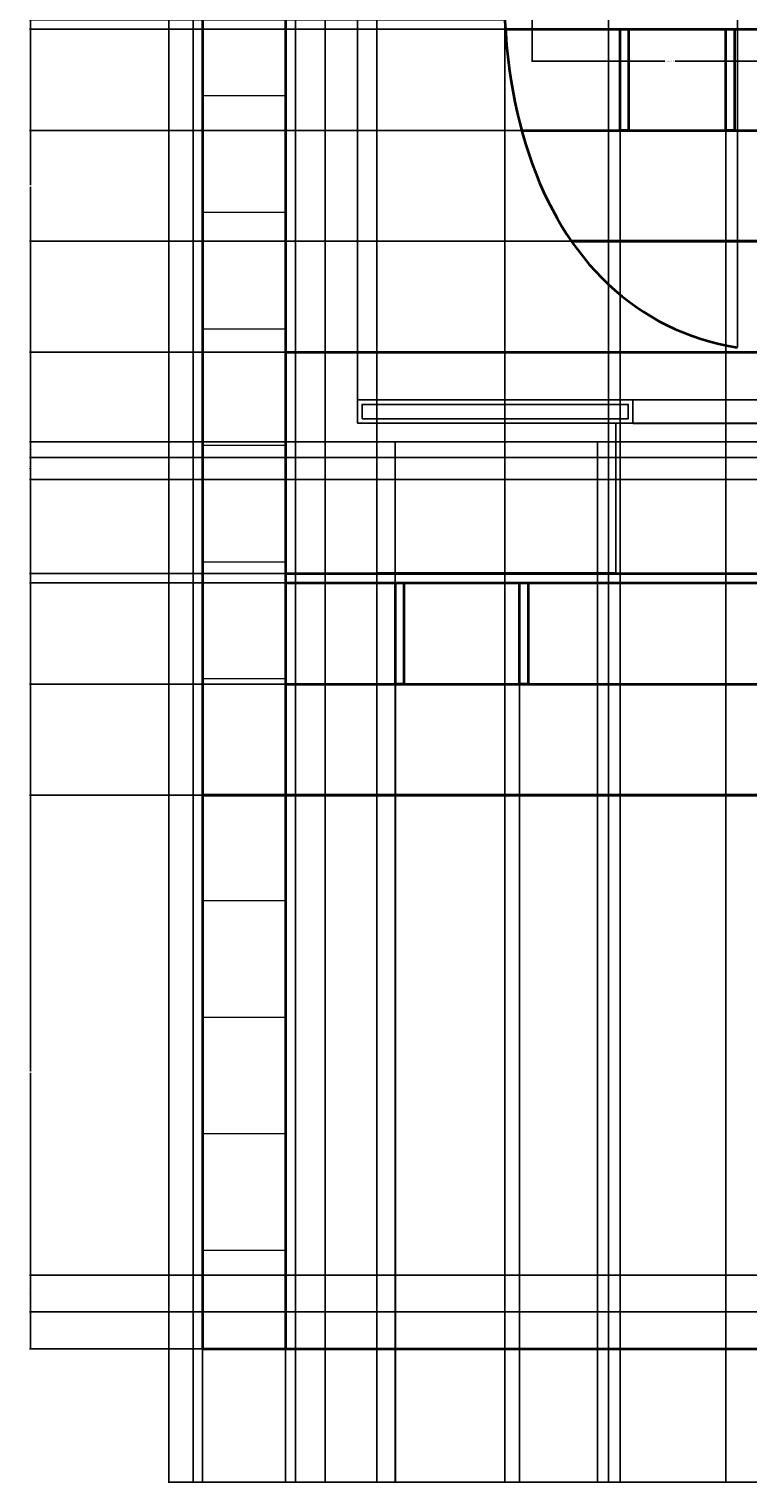
# Model space of a CAD drawing. Units: inches. Extents: x -19 to 408, y -26 to 603.
# Tile 1 of 7: x -19 to 137, y -26 to 289. Entities that reach past the tile are written whole.
import ezdxf

# ---------------------------------------------------------------- set-up
doc = ezdxf.new("R2010")
doc.units = ezdxf.units.IN
doc.header["$MEASUREMENT"] = 0
for name, color, linetype, lineweight in [('A-ANNO-DIMS', 2, 'Continuous', 18), ('A-ELEV', 7, 'Continuous', 35), ('A-GLAZ', 4, 'Continuous', 25), ('A-WALL-PATT', 8, 'Continuous', 13)]:
    doc.layers.add(name, color=color, linetype=linetype, lineweight=lineweight)
doc.styles.get("Standard").update_dxf_attribs({"font": 'arial.ttf'})
doc.dimstyles.get("Standard").update_dxf_attribs({"dimtxt": 0.18, "dimasz": 0.18, "dimexe": 0.18, "dimexo": 0.0625, "dimgap": 0.09, "dimtad": 0, "dimtih": 1, "dimtoh": 1, "dimdec": 4, "dimzin": 0, "dimdsep": 46, "dimtxsty": 'Standard', "dimcen": 0.09, "dimadec": 0, "dimazin": 0, "dimtfac": 1, "dimtdec": 4, "dimtofl": 0, "dimtmove": 0, "dimatfit": 3, "dimfxl": 1, "dimtolj": 1, "dimtzin": 0, "dimarcsym": 0})

# ---------------------------------------------------------------- blocks, each defined once
blk = doc.blocks.new('WIN-1200')
for points in [[(0, 32.56), (59.66, 32.56), (59.66, 37.64), (0, 37.64)], [(1, 33.56), (58.66, 33.56), (58.66, 36.64), (1, 36.64)]]:
    blk.add_lwpolyline(points, close=True)
for points in [[(4.17, 0), (4.17, 32.56), (55.99, 32.56), (55.99, 0)], [(8.17, 0), (8.17, 28.56), (51.99, 28.56), (51.99, 0)]]:
    blk.add_lwpolyline(points)
blk = doc.blocks.new('RAIL-POST')
blk.add_lwpolyline([(0, 22), (1.83, 22), (1.83, 0), (0, 0)], close=True)
blk = doc.blocks.new('*D4')
at = {"layer": 'A-ANNO-DIMS', "color": 0, "lineweight": -2, "transparency": 16777216}
for p, q in [((89.99, 291.08), (89.99, 282.02)), ((149.65, 291.08), (149.65, 282.02)), ((90.17, 282.2), (118.7, 282.2)), ((149.47, 282.2), (120.94, 282.2))]:
    blk.add_line(p, q, dxfattribs=at)
at = {"layer": 'A-ANNO-DIMS', "color": 0, "transparency": 16777216}
for points in [[(90.17, 282.23), (90.17, 282.17), (89.99, 282.2)], [(149.47, 282.23), (149.47, 282.17), (149.65, 282.2)]]:
    blk.add_solid(points, dxfattribs=at)
at = {"layer": 'Defpoints', "color": 0, "transparency": 16777216}
for p in [(89.99, 291.15), (149.65, 291.15), (149.65, 282.2)]:
    blk.add_point(p, dxfattribs=at)
at = {"layer": 'A-ANNO-DIMS', "color": 0, "transparency": 16777216, "insert": (119.82, 282.2), "char_height": 0.18, "attachment_point": 5}
blk.add_mtext('\\A1;WINDOW 60 TYP.', dxfattribs=at)
blk = doc.blocks.new('*D10')
at = {"layer": 'A-ANNO-DIMS', "color": 0, "lineweight": -2, "transparency": 16777216}
for p, q in [((18.57, 3.08), (18.57, -25.93)), ((36.57, 3.08), (36.57, -25.93)), ((18.75, -25.75), (27.36, -25.75)), ((36.39, -25.75), (27.78, -25.75))]:
    blk.add_line(p, q, dxfattribs=at)
at = {"layer": 'A-ANNO-DIMS', "color": 0, "transparency": 16777216}
for points in [[(18.75, -25.72), (18.75, -25.78), (18.57, -25.75)], [(36.39, -25.72), (36.39, -25.78), (36.57, -25.75)]]:
    blk.add_solid(points, dxfattribs=at)
at = {"layer": 'Defpoints', "color": 0, "transparency": 16777216}
for p in [(18.57, 3.15), (36.57, 3.15), (36.57, -25.75)]:
    blk.add_point(p, dxfattribs=at)
at = {"layer": 'A-ANNO-DIMS', "color": 0, "transparency": 16777216, "insert": (27.57, -25.75), "char_height": 0.18, "attachment_point": 5}
blk.add_mtext('\\A1;18', dxfattribs=at)
blk = doc.blocks.new('*D11')
at = {"layer": 'A-ANNO-DIMS', "color": 0, "lineweight": -2, "transparency": 16777216}
for p, q in [((150.57, 123.08), (150.57, -25.93)), ((36.57, 3.08), (36.57, -25.93)), ((36.75, -25.75), (93.29, -25.75)), ((150.39, -25.75), (93.85, -25.75))]:
    blk.add_line(p, q, dxfattribs=at)
at = {"layer": 'A-ANNO-DIMS', "color": 0, "transparency": 16777216}
for points in [[(36.75, -25.72), (36.75, -25.78), (36.57, -25.75)], [(150.39, -25.72), (150.39, -25.78), (150.57, -25.75)]]:
    blk.add_solid(points, dxfattribs=at)
at = {"layer": 'Defpoints', "color": 0, "transparency": 16777216}
for p in [(150.57, 123.15), (36.57, 3.15), (150.57, -25.75)]:
    blk.add_point(p, dxfattribs=at)
at = {"layer": 'A-ANNO-DIMS', "color": 0, "transparency": 16777216, "insert": (93.57, -25.75), "char_height": 0.18, "attachment_point": 5}
blk.add_mtext('\\A1;114', dxfattribs=at)
blk = doc.blocks.new('*D17')
at = {"layer": 'A-ANNO-DIMS', "color": 0, "lineweight": -2, "transparency": 16777216}
for p, q in [((18.51, 123.15), (-18.88, 123.15)), ((-18.7, 122.97), (-18.7, 63.33)), ((-18.7, 3.33), (-18.7, 62.97)), ((18.51, 3.15), (-18.88, 3.15))]:
    blk.add_line(p, q, dxfattribs=at)
at = {"layer": 'A-ANNO-DIMS', "color": 0, "transparency": 16777216}
for points in [[(-18.73, 122.97), (-18.67, 122.97), (-18.7, 123.15)], [(-18.73, 3.33), (-18.67, 3.33), (-18.7, 3.15)]]:
    blk.add_solid(points, dxfattribs=at)
at = {"layer": 'Defpoints', "color": 0, "transparency": 16777216}
for p in [(-18.7, 123.15), (18.57, 123.15), (18.57, 3.15)]:
    blk.add_point(p, dxfattribs=at)
at = {"layer": 'A-ANNO-DIMS', "color": 0, "transparency": 16777216, "insert": (-18.7, 63.15), "char_height": 0.18, "attachment_point": 5}
blk.add_mtext('\\A1;120', dxfattribs=at)
blk = doc.blocks.new('*D18')
at = {"layer": 'A-ANNO-DIMS', "color": 0, "lineweight": -2, "transparency": 16777216}
for p, q in [((36.51, 219.15), (-18.88, 219.15)), ((-18.7, 218.97), (-18.7, 171.33)), ((-18.7, 123.33), (-18.7, 170.97)), ((18.51, 123.15), (-18.88, 123.15))]:
    blk.add_line(p, q, dxfattribs=at)
at = {"layer": 'A-ANNO-DIMS', "color": 0, "transparency": 16777216}
for points in [[(-18.73, 218.97), (-18.67, 218.97), (-18.7, 219.15)], [(-18.73, 123.33), (-18.67, 123.33), (-18.7, 123.15)]]:
    blk.add_solid(points, dxfattribs=at)
at = {"layer": 'Defpoints', "color": 0, "transparency": 16777216}
for p in [(-18.7, 219.15), (36.57, 219.15), (18.57, 123.15)]:
    blk.add_point(p, dxfattribs=at)
at = {"layer": 'A-ANNO-DIMS', "color": 0, "transparency": 16777216, "insert": (-18.7, 171.15), "char_height": 0.18, "attachment_point": 5}
blk.add_mtext('\\A1;96', dxfattribs=at)
blk = doc.blocks.new('*D19')
at = {"layer": 'A-ANNO-DIMS', "color": 0, "lineweight": -2, "transparency": 16777216}
for p, q in [((84.02, 291.15), (-18.88, 291.15)), ((-18.7, 290.97), (-18.7, 255.33)), ((-18.7, 219.33), (-18.7, 254.97)), ((36.51, 219.15), (-18.88, 219.15))]:
    blk.add_line(p, q, dxfattribs=at)
at = {"layer": 'A-ANNO-DIMS', "color": 0, "transparency": 16777216}
for points in [[(-18.73, 290.97), (-18.67, 290.97), (-18.7, 291.15)], [(-18.73, 219.33), (-18.67, 219.33), (-18.7, 219.15)]]:
    blk.add_solid(points, dxfattribs=at)
at = {"layer": 'Defpoints', "color": 0, "transparency": 16777216}
for p in [(-18.7, 291.15), (84.08, 291.15), (36.57, 219.15)]:
    blk.add_point(p, dxfattribs=at)
at = {"layer": 'A-ANNO-DIMS', "color": 0, "transparency": 16777216, "insert": (-18.7, 255.15), "char_height": 0.18, "attachment_point": 5}
blk.add_mtext('\\A1;72', dxfattribs=at)
blk = doc.blocks.new('*D33')
at = {"layer": 'A-ANNO-DIMS', "color": 0, "lineweight": -2, "transparency": 16777216}
for p, q in [((36.51, 169.15), (-18.88, 169.15)), ((-18.7, 168.97), (-18.7, 158.33)), ((-18.7, 147.33), (-18.7, 157.97)), ((36.51, 147.15), (-18.88, 147.15))]:
    blk.add_line(p, q, dxfattribs=at)
at = {"layer": 'A-ANNO-DIMS', "color": 0, "transparency": 16777216}
for points in [[(-18.73, 168.97), (-18.67, 168.97), (-18.7, 169.15)], [(-18.73, 147.33), (-18.67, 147.33), (-18.7, 147.15)]]:
    blk.add_solid(points, dxfattribs=at)
at = {"layer": 'Defpoints', "color": 0, "transparency": 16777216}
for p in [(-18.7, 169.15), (36.57, 169.15), (36.57, 147.15)]:
    blk.add_point(p, dxfattribs=at)
at = {"layer": 'A-ANNO-DIMS', "color": 0, "transparency": 16777216, "insert": (-18.7, 158.15), "char_height": 0.18, "attachment_point": 5}
blk.add_mtext('\\A1;22', dxfattribs=at)
blk = doc.blocks.new('*D34')
at = {"layer": 'A-ANNO-DIMS', "color": 0, "lineweight": -2, "transparency": 16777216}
for p, q in [((36.51, 171.15), (-18.88, 171.15)), ((-18.7, 170.97), (-18.7, 170.33)), ((36.51, 169.15), (-18.88, 169.15)), ((-18.7, 169.33), (-18.7, 169.97))]:
    blk.add_line(p, q, dxfattribs=at)
at = {"layer": 'A-ANNO-DIMS', "color": 0, "transparency": 16777216}
for points in [[(-18.73, 170.97), (-18.67, 170.97), (-18.7, 171.15)], [(-18.73, 169.33), (-18.67, 169.33), (-18.7, 169.15)]]:
    blk.add_solid(points, dxfattribs=at)
at = {"layer": 'Defpoints', "color": 0, "transparency": 16777216}
for p in [(-18.7, 171.15), (36.57, 171.15), (36.57, 169.15)]:
    blk.add_point(p, dxfattribs=at)
at = {"layer": 'A-ANNO-DIMS', "color": 0, "transparency": 16777216, "insert": (-18.7, 170.15), "char_height": 0.18, "attachment_point": 5}
blk.add_mtext('\\A1;2', dxfattribs=at)
blk = doc.blocks.new('*D35')
at = {"layer": 'A-ANNO-DIMS', "color": 0, "lineweight": -2, "transparency": 16777216}
for p, q in [((36.57, 171.21), (36.57, 602.9)), ((36.75, 602.72), (43.91, 602.72)), ((51.97, 602.72), (44.82, 602.72)), ((52.15, 203.77), (52.15, 602.9))]:
    blk.add_line(p, q, dxfattribs=at)
at = {"layer": 'A-ANNO-DIMS', "color": 0, "transparency": 16777216}
for points in [[(36.75, 602.75), (36.75, 602.69), (36.57, 602.72)], [(51.97, 602.75), (51.97, 602.69), (52.15, 602.72)]]:
    blk.add_solid(points, dxfattribs=at)
at = {"layer": 'Defpoints', "color": 0, "transparency": 16777216}
for p in [(52.15, 602.72), (52.15, 203.7), (36.57, 171.15)]:
    blk.add_point(p, dxfattribs=at)
at = {"layer": 'A-ANNO-DIMS', "color": 0, "transparency": 16777216, "insert": (44.36, 602.72), "char_height": 0.18, "attachment_point": 5}
blk.add_mtext('\\A1;15.582', dxfattribs=at)
blk = doc.blocks.new('*D36')
at = {"layer": 'A-ANNO-DIMS', "color": 0, "lineweight": -2, "transparency": 16777216}
for p, q in [((52.15, 203.77), (52.15, 602.9)), ((52.33, 602.72), (96.69, 602.72)), ((141.84, 602.72), (97.48, 602.72)), ((142.02, 171.21), (142.02, 602.9))]:
    blk.add_line(p, q, dxfattribs=at)
at = {"layer": 'A-ANNO-DIMS', "color": 0, "transparency": 16777216}
for points in [[(52.33, 602.75), (52.33, 602.69), (52.15, 602.72)], [(141.84, 602.75), (141.84, 602.69), (142.02, 602.72)]]:
    blk.add_solid(points, dxfattribs=at)
at = {"layer": 'Defpoints', "color": 0, "transparency": 16777216}
for p in [(142.02, 602.72), (52.15, 203.7), (142.02, 171.15)]:
    blk.add_point(p, dxfattribs=at)
at = {"layer": 'A-ANNO-DIMS', "color": 0, "transparency": 16777216, "insert": (97.09, 602.72), "char_height": 0.18, "attachment_point": 5}
blk.add_mtext('\\A1;89.87', dxfattribs=at)
blk = doc.blocks.new('*D39')
at = {"layer": 'A-ANNO-DIMS', "color": 0, "lineweight": -2, "transparency": 16777216}
for p, q in [((36.57, 147.08), (36.57, -25.93)), ((60.39, 147.08), (60.39, -25.93)), ((36.75, -25.75), (48.01, -25.75)), ((60.21, -25.75), (48.94, -25.75))]:
    blk.add_line(p, q, dxfattribs=at)
at = {"layer": 'A-ANNO-DIMS', "color": 0, "transparency": 16777216}
for points in [[(36.75, -25.72), (36.75, -25.78), (36.57, -25.75)], [(60.21, -25.72), (60.21, -25.78), (60.39, -25.75)]]:
    blk.add_solid(points, dxfattribs=at)
at = {"layer": 'Defpoints', "color": 0, "transparency": 16777216}
for p in [(36.57, 147.15), (60.39, 147.15), (60.39, -25.75)]:
    blk.add_point(p, dxfattribs=at)
at = {"layer": 'A-ANNO-DIMS', "color": 0, "transparency": 16777216, "insert": (48.48, -25.75), "char_height": 0.18, "attachment_point": 5}
blk.add_mtext('\\A1;23.815', dxfattribs=at)
blk = doc.blocks.new('*D40')
at = {"layer": 'A-ANNO-DIMS', "color": 0, "lineweight": -2, "transparency": 16777216}
for p, q in [((60.39, 147.08), (60.39, -25.93)), ((87.25, 147.08), (87.25, -25.93)), ((60.57, -25.75), (73.42, -25.75)), ((87.07, -25.75), (74.22, -25.75))]:
    blk.add_line(p, q, dxfattribs=at)
at = {"layer": 'A-ANNO-DIMS', "color": 0, "transparency": 16777216}
for points in [[(60.57, -25.72), (60.57, -25.78), (60.39, -25.75)], [(87.07, -25.72), (87.07, -25.78), (87.25, -25.75)]]:
    blk.add_solid(points, dxfattribs=at)
at = {"layer": 'Defpoints', "color": 0, "transparency": 16777216}
for p in [(60.39, 147.15), (87.25, 147.15), (87.25, -25.75)]:
    blk.add_point(p, dxfattribs=at)
at = {"layer": 'A-ANNO-DIMS', "color": 0, "transparency": 16777216, "insert": (73.82, -25.75), "char_height": 0.18, "attachment_point": 5}
blk.add_mtext('\\A1;26.87', dxfattribs=at)
blk = doc.blocks.new('*D41')
at = {"layer": 'A-ANNO-DIMS', "color": 0, "lineweight": -2, "transparency": 16777216}
for p, q in [((87.25, 147.08), (87.25, -25.93)), ((150.62, 147.08), (150.62, -25.93)), ((87.43, -25.75), (118.54, -25.75)), ((150.44, -25.75), (119.33, -25.75))]:
    blk.add_line(p, q, dxfattribs=at)
at = {"layer": 'A-ANNO-DIMS', "color": 0, "transparency": 16777216}
for points in [[(87.43, -25.72), (87.43, -25.78), (87.25, -25.75)], [(150.44, -25.72), (150.44, -25.78), (150.62, -25.75)]]:
    blk.add_solid(points, dxfattribs=at)
at = {"layer": 'Defpoints', "color": 0, "transparency": 16777216}
for p in [(87.25, 147.15), (150.62, 147.15), (150.62, -25.75)]:
    blk.add_point(p, dxfattribs=at)
at = {"layer": 'A-ANNO-DIMS', "color": 0, "transparency": 16777216, "insert": (118.93, -25.75), "char_height": 0.18, "attachment_point": 5}
blk.add_mtext('\\A1;63.36', dxfattribs=at)
blk = doc.blocks.new('*D45')
at = {"layer": 'A-ANNO-DIMS', "color": 0, "lineweight": -2, "transparency": 16777216}
for p, q in [((36.57, 219.21), (36.57, 602.9)), ((36.75, 602.72), (85.2, 602.72)), ((134.3, 602.72), (85.85, 602.72)), ((134.48, 220.21), (134.48, 602.9))]:
    blk.add_line(p, q, dxfattribs=at)
at = {"layer": 'A-ANNO-DIMS', "color": 0, "transparency": 16777216}
for points in [[(36.75, 602.75), (36.75, 602.69), (36.57, 602.72)], [(134.3, 602.75), (134.3, 602.69), (134.48, 602.72)]]:
    blk.add_solid(points, dxfattribs=at)
at = {"layer": 'Defpoints', "color": 0, "transparency": 16777216}
for p in [(134.48, 602.72), (36.57, 219.15), (134.48, 220.15)]:
    blk.add_point(p, dxfattribs=at)
at = {"layer": 'A-ANNO-DIMS', "color": 0, "transparency": 16777216, "insert": (85.52, 602.72), "char_height": 0.18, "attachment_point": 5}
blk.add_mtext('\\A1;97.9', dxfattribs=at)
blk = doc.blocks.new('*D47')
at = {"layer": 'A-ANNO-DIMS', "color": 0, "lineweight": -2, "transparency": 16777216}
for p, q in [((52.15, 203.77), (52.15, 602.9)), ((52.33, 602.72), (53.84, 602.72)), ((56.15, 602.72), (54.64, 602.72)), ((56.33, 203.77), (56.33, 602.9))]:
    blk.add_line(p, q, dxfattribs=at)
at = {"layer": 'A-ANNO-DIMS', "color": 0, "transparency": 16777216}
for points in [[(52.33, 602.75), (52.33, 602.69), (52.15, 602.72)], [(56.15, 602.75), (56.15, 602.69), (56.33, 602.72)]]:
    blk.add_solid(points, dxfattribs=at)
at = {"layer": 'Defpoints', "color": 0, "transparency": 16777216}
for p in [(56.33, 602.72), (52.15, 203.7), (56.33, 203.7)]:
    blk.add_point(p, dxfattribs=at)
at = {"layer": 'A-ANNO-DIMS', "color": 0, "transparency": 16777216, "insert": (54.24, 602.72), "char_height": 0.18, "attachment_point": 5}
blk.add_mtext('\\A1;4.173', dxfattribs=at)
blk = doc.blocks.new('*D48')
at = {"layer": 'A-ANNO-DIMS', "color": 0, "lineweight": -2, "transparency": 16777216}
for p, q in [((56.33, 171.08), (56.33, -25.93)), ((60.33, 171.08), (60.33, -25.93)), ((56.51, -25.75), (58.17, -25.75)), ((60.15, -25.75), (58.48, -25.75))]:
    blk.add_line(p, q, dxfattribs=at)
at = {"layer": 'A-ANNO-DIMS', "color": 0, "transparency": 16777216}
for points in [[(56.51, -25.72), (56.51, -25.78), (56.33, -25.75)], [(60.15, -25.72), (60.15, -25.78), (60.33, -25.75)]]:
    blk.add_solid(points, dxfattribs=at)
at = {"layer": 'Defpoints', "color": 0, "transparency": 16777216}
for p in [(56.33, 171.15), (60.33, 171.15), (60.33, -25.75)]:
    blk.add_point(p, dxfattribs=at)
at = {"layer": 'A-ANNO-DIMS', "color": 0, "transparency": 16777216, "insert": (58.33, -25.75), "char_height": 0.18, "attachment_point": 5}
blk.add_mtext('\\A1;4', dxfattribs=at)
blk = doc.blocks.new('*D49')
at = {"layer": 'A-ANNO-DIMS', "color": 0, "lineweight": -2, "transparency": 16777216}
for p, q in [((60.33, 171.08), (60.33, -25.93)), ((104.14, 171.08), (104.14, -25.93)), ((60.51, -25.75), (81.84, -25.75)), ((103.96, -25.75), (82.63, -25.75))]:
    blk.add_line(p, q, dxfattribs=at)
at = {"layer": 'A-ANNO-DIMS', "color": 0, "transparency": 16777216}
for points in [[(60.51, -25.72), (60.51, -25.78), (60.33, -25.75)], [(103.96, -25.72), (103.96, -25.78), (104.14, -25.75)]]:
    blk.add_solid(points, dxfattribs=at)
at = {"layer": 'Defpoints', "color": 0, "transparency": 16777216}
for p in [(60.33, 171.15), (104.14, 171.15), (104.14, -25.75)]:
    blk.add_point(p, dxfattribs=at)
at = {"layer": 'A-ANNO-DIMS', "color": 0, "transparency": 16777216, "insert": (82.24, -25.75), "char_height": 0.18, "attachment_point": 5}
blk.add_mtext('\\A1;43.82', dxfattribs=at)
blk = doc.blocks.new('*D50')
at = {"layer": 'A-ANNO-DIMS', "color": 0, "lineweight": -2, "transparency": 16777216}
for p, q in [((104.21, 199.7), (407.65, 199.7)), ((407.47, 199.52), (407.47, 185.61)), ((407.47, 171.33), (407.47, 185.24)), ((104.21, 171.15), (407.65, 171.15))]:
    blk.add_line(p, q, dxfattribs=at)
at = {"layer": 'A-ANNO-DIMS', "color": 0, "transparency": 16777216}
for points in [[(407.44, 199.52), (407.5, 199.52), (407.47, 199.7)], [(407.44, 171.33), (407.5, 171.33), (407.47, 171.15)]]:
    blk.add_solid(points, dxfattribs=at)
at = {"layer": 'Defpoints', "color": 0, "transparency": 16777216}
for p in [(104.14, 199.7), (407.47, 199.7), (104.14, 171.15)]:
    blk.add_point(p, dxfattribs=at)
at = {"layer": 'A-ANNO-DIMS', "color": 0, "transparency": 16777216, "insert": (407.47, 185.43), "char_height": 0.18, "attachment_point": 5}
blk.add_mtext('\\A1;28.557', dxfattribs=at)
blk = doc.blocks.new('*D51')
at = {"layer": 'A-ANNO-DIMS', "color": 0, "lineweight": -2, "transparency": 16777216}
for p, q in [((108.207069, 203.703989), (407.651202, 203.703989)), ((407.471202, 203.523989), (407.471202, 201.883989)), ((104.207069, 199.703989), (407.651202, 199.703989)), ((407.471202, 199.883989), (407.471202, 201.523989))]:
    blk.add_line(p, q, dxfattribs=at)
at = {"layer": 'A-ANNO-DIMS', "color": 0, "transparency": 16777216}
for points in [[(407.441202, 203.523989), (407.501202, 203.523989), (407.471202, 203.703989)], [(407.441202, 199.883989), (407.501202, 199.883989), (407.471202, 199.703989)]]:
    blk.add_solid(points, dxfattribs=at)
at = {"layer": 'Defpoints', "color": 0, "transparency": 16777216}
for p in [(108.144569, 203.703989), (407.471202, 203.703989), (104.144569, 199.703989)]:
    blk.add_point(p, dxfattribs=at)
at = {"layer": 'A-ANNO-DIMS', "color": 0, "transparency": 16777216, "insert": (407.471202, 201.703989), "char_height": 0.18, "attachment_point": 5}
blk.add_mtext('\\A1;4', dxfattribs=at)
blk = doc.blocks.new('*D52')
at = {"layer": 'A-ANNO-DIMS', "color": 0, "lineweight": -2, "transparency": 16777216}
for p, q in [((111.87, 208.79), (407.65, 208.79)), ((407.47, 208.61), (407.47, 206.43)), ((407.47, 203.88), (407.47, 206.07)), ((111.87, 203.7), (407.65, 203.7))]:
    blk.add_line(p, q, dxfattribs=at)
at = {"layer": 'A-ANNO-DIMS', "color": 0, "transparency": 16777216}
for points in [[(407.44, 208.61), (407.5, 208.61), (407.47, 208.79)], [(407.44, 203.88), (407.5, 203.88), (407.47, 203.7)]]:
    blk.add_solid(points, dxfattribs=at)
at = {"layer": 'Defpoints', "color": 0, "transparency": 16777216}
for p in [(111.81, 208.79), (407.47, 208.79), (111.81, 203.7)]:
    blk.add_point(p, dxfattribs=at)
at = {"layer": 'A-ANNO-DIMS', "color": 0, "transparency": 16777216, "insert": (407.47, 206.25), "char_height": 0.18, "attachment_point": 5}
blk.add_mtext('\\A1;5.086', dxfattribs=at)
blk = doc.blocks.new('*D57')
at = {"layer": 'A-ANNO-DIMS', "color": 0, "lineweight": -2, "transparency": 16777216}
for p, q in [((148.99, 196.31), (-18.88, 196.31)), ((-18.7, 196.13), (-18.7, 194.11)), ((-18.7, 191.73), (-18.7, 193.75)), ((148.99, 191.55), (-18.88, 191.55))]:
    blk.add_line(p, q, dxfattribs=at)
at = {"layer": 'A-ANNO-DIMS', "color": 0, "transparency": 16777216}
for points in [[(-18.73, 196.13), (-18.67, 196.13), (-18.7, 196.31)], [(-18.73, 191.73), (-18.67, 191.73), (-18.7, 191.55)]]:
    blk.add_solid(points, dxfattribs=at)
at = {"layer": 'Defpoints', "color": 0, "transparency": 16777216}
for p in [(-18.7, 196.31), (149.05, 196.31), (149.05, 191.55)]:
    blk.add_point(p, dxfattribs=at)
at = {"layer": 'A-ANNO-DIMS', "color": 0, "transparency": 16777216, "insert": (-18.7, 193.93), "char_height": 0.18, "attachment_point": 5}
blk.add_mtext('\\A1;4.756', dxfattribs=at)
blk = doc.blocks.new('*D58')
at = {"layer": 'A-ANNO-DIMS', "color": 0, "lineweight": -2, "transparency": 16777216}
for p, q in [((145.96, 199.7), (-18.88, 199.7)), ((-18.7, 199.52), (-18.7, 198.19)), ((148.99, 196.31), (-18.88, 196.31)), ((-18.7, 196.49), (-18.7, 197.82))]:
    blk.add_line(p, q, dxfattribs=at)
at = {"layer": 'A-ANNO-DIMS', "color": 0, "transparency": 16777216}
for points in [[(-18.73, 199.52), (-18.67, 199.52), (-18.7, 199.7)], [(-18.73, 196.49), (-18.67, 196.49), (-18.7, 196.31)]]:
    blk.add_solid(points, dxfattribs=at)
at = {"layer": 'Defpoints', "color": 0, "transparency": 16777216}
for p in [(-18.7, 199.7), (146.02, 199.7), (149.05, 196.31)]:
    blk.add_point(p, dxfattribs=at)
at = {"layer": 'A-ANNO-DIMS', "color": 0, "transparency": 16777216, "insert": (-18.7, 198), "char_height": 0.18, "attachment_point": 5}
blk.add_mtext('\\A1;3.398', dxfattribs=at)
blk = doc.blocks.new('*D60')
at = {"layer": 'A-ANNO-DIMS', "color": 0, "lineweight": -2, "transparency": 16777216}
for p, q in [((84.08, 291.08), (84.08, -25.93)), ((109.02, 267.08), (109.02, -25.93)), ((84.26, -25.75), (96.15, -25.75)), ((108.84, -25.75), (96.94, -25.75))]:
    blk.add_line(p, q, dxfattribs=at)
at = {"layer": 'A-ANNO-DIMS', "color": 0, "transparency": 16777216}
for points in [[(84.26, -25.72), (84.26, -25.78), (84.08, -25.75)], [(108.84, -25.72), (108.84, -25.78), (109.02, -25.75)]]:
    blk.add_solid(points, dxfattribs=at)
at = {"layer": 'Defpoints', "color": 0, "transparency": 16777216}
for p in [(84.08, 291.15), (109.02, 267.15), (109.02, -25.75)]:
    blk.add_point(p, dxfattribs=at)
at = {"layer": 'A-ANNO-DIMS', "color": 0, "transparency": 16777216, "insert": (96.55, -25.75), "char_height": 0.18, "attachment_point": 5}
blk.add_mtext('\\A1;24.94', dxfattribs=at)
blk = doc.blocks.new('*D61')
at = {"layer": 'A-ANNO-DIMS', "color": 0, "lineweight": -2, "transparency": 16777216}
for p, q in [((109.02, 267.08), (109.02, -25.93)), ((131.96, 267.08), (131.96, -25.93)), ((109.2, -25.75), (120.02, -25.75)), ((131.78, -25.75), (120.95, -25.75))]:
    blk.add_line(p, q, dxfattribs=at)
at = {"layer": 'A-ANNO-DIMS', "color": 0, "transparency": 16777216}
for points in [[(109.2, -25.72), (109.2, -25.78), (109.02, -25.75)], [(131.78, -25.72), (131.78, -25.78), (131.96, -25.75)]]:
    blk.add_solid(points, dxfattribs=at)
at = {"layer": 'Defpoints', "color": 0, "transparency": 16777216}
for p in [(109.02, 267.15), (131.96, 267.15), (131.96, -25.75)]:
    blk.add_point(p, dxfattribs=at)
at = {"layer": 'A-ANNO-DIMS', "color": 0, "transparency": 16777216, "insert": (120.49, -25.75), "char_height": 0.18, "attachment_point": 5}
blk.add_mtext('\\A1;22.944', dxfattribs=at)
blk = doc.blocks.new('*D62')
at = {"layer": 'A-ANNO-DIMS', "color": 0, "lineweight": -2, "transparency": 16777216}
for p, q in [((131.96, 267.08), (131.96, -25.93)), ((185.68, 267.08), (185.68, -25.93)), ((132.14, -25.75), (158.43, -25.75)), ((185.5, -25.75), (159.21, -25.75))]:
    blk.add_line(p, q, dxfattribs=at)
at = {"layer": 'A-ANNO-DIMS', "color": 0, "transparency": 16777216}
for points in [[(132.14, -25.72), (132.14, -25.78), (131.96, -25.75)], [(185.5, -25.72), (185.5, -25.78), (185.68, -25.75)]]:
    blk.add_solid(points, dxfattribs=at)
at = {"layer": 'Defpoints', "color": 0, "transparency": 16777216}
for p in [(131.96, 267.15), (185.68, 267.15), (185.68, -25.75)]:
    blk.add_point(p, dxfattribs=at)
at = {"layer": 'A-ANNO-DIMS', "color": 0, "transparency": 16777216, "insert": (158.82, -25.75), "char_height": 0.18, "attachment_point": 5}
blk.add_mtext('\\A1;53.72', dxfattribs=at)
blk = doc.blocks.new('*D67')
at = {"layer": 'A-ANNO-DIMS', "color": 0, "lineweight": -2, "transparency": 16777216}
for p, q in [((87.66, 267.15), (-18.88, 267.15)), ((-18.7, 266.97), (-18.7, 255.33)), ((-18.7, 243.33), (-18.7, 254.97)), ((98.46, 243.15), (-18.88, 243.15))]:
    blk.add_line(p, q, dxfattribs=at)
at = {"layer": 'A-ANNO-DIMS', "color": 0, "transparency": 16777216}
for points in [[(-18.73, 266.97), (-18.67, 266.97), (-18.7, 267.15)], [(-18.73, 243.33), (-18.67, 243.33), (-18.7, 243.15)]]:
    blk.add_solid(points, dxfattribs=at)
at = {"layer": 'Defpoints', "color": 0, "transparency": 16777216}
for p in [(-18.7, 267.15), (87.72, 267.15), (98.52, 243.15)]:
    blk.add_point(p, dxfattribs=at)
at = {"layer": 'A-ANNO-DIMS', "color": 0, "transparency": 16777216, "insert": (-18.7, 255.15), "char_height": 0.18, "attachment_point": 5}
blk.add_mtext('\\A1;24', dxfattribs=at)
blk = doc.blocks.new('*D68')
at = {"layer": 'A-ANNO-DIMS', "color": 0, "lineweight": -2, "transparency": 16777216}
for p, q in [((84.13, 289.15), (-18.88, 289.15)), ((-18.7, 288.97), (-18.7, 278.33)), ((-18.7, 267.33), (-18.7, 277.97)), ((87.66, 267.15), (-18.88, 267.15))]:
    blk.add_line(p, q, dxfattribs=at)
at = {"layer": 'A-ANNO-DIMS', "color": 0, "transparency": 16777216}
for points in [[(-18.73, 288.97), (-18.67, 288.97), (-18.7, 289.15)], [(-18.73, 267.33), (-18.67, 267.33), (-18.7, 267.15)]]:
    blk.add_solid(points, dxfattribs=at)
at = {"layer": 'Defpoints', "color": 0, "transparency": 16777216}
for p in [(-18.7, 289.15), (84.19, 289.15), (87.72, 267.15)]:
    blk.add_point(p, dxfattribs=at)
at = {"layer": 'A-ANNO-DIMS', "color": 0, "transparency": 16777216, "insert": (-18.7, 278.15), "char_height": 0.18, "attachment_point": 5}
blk.add_mtext('\\A1;22', dxfattribs=at)
blk = doc.blocks.new('*D94')
at = {"layer": 'A-ANNO-DIMS', "color": 0, "lineweight": -2, "transparency": 16777216}
for p, q in [((150.51, 19.1), (-18.88, 19.1)), ((-18.7, 18.92), (-18.7, 15.32)), ((-18.7, 11.36), (-18.7, 14.96)), ((150.51, 11.18), (-18.88, 11.18))]:
    blk.add_line(p, q, dxfattribs=at)
at = {"layer": 'A-ANNO-DIMS', "color": 0, "transparency": 16777216}
for points in [[(-18.73, 18.92), (-18.67, 18.92), (-18.7, 19.1)], [(-18.73, 11.36), (-18.67, 11.36), (-18.7, 11.18)]]:
    blk.add_solid(points, dxfattribs=at)
at = {"layer": 'Defpoints', "color": 0, "transparency": 16777216}
for p in [(-18.7, 19.1), (150.57, 19.1), (150.57, 11.18)]:
    blk.add_point(p, dxfattribs=at)
at = {"layer": 'A-ANNO-DIMS', "color": 0, "transparency": 16777216, "insert": (-18.7, 15.14), "char_height": 0.18, "attachment_point": 5}
blk.add_mtext('\\A1;7.919', dxfattribs=at)
blk = doc.blocks.new('*D99')
at = {"layer": 'A-ANNO-DIMS', "color": 0, "lineweight": -2, "transparency": 16777216}
for p, q in [((11.24, 569.54), (11.24, -25.93)), ((45.11, 569.54), (45.11, -25.93)), ((11.42, -25.75), (27.71, -25.75)), ((44.93, -25.75), (28.64, -25.75))]:
    blk.add_line(p, q, dxfattribs=at)
at = {"layer": 'A-ANNO-DIMS', "color": 0, "transparency": 16777216}
for points in [[(11.42, -25.72), (11.42, -25.78), (11.24, -25.75)], [(44.93, -25.72), (44.93, -25.78), (45.11, -25.75)]]:
    blk.add_solid(points, dxfattribs=at)
at = {"layer": 'Defpoints', "color": 0, "transparency": 16777216}
for p in [(11.24, 569.61), (45.11, 569.61), (45.11, -25.75)]:
    blk.add_point(p, dxfattribs=at)
at = {"layer": 'A-ANNO-DIMS', "color": 0, "transparency": 16777216, "insert": (28.17, -25.75), "char_height": 0.18, "attachment_point": 5}
blk.add_mtext('\\A1;33.876', dxfattribs=at)
blk = doc.blocks.new('*D101')
at = {"layer": 'A-ANNO-DIMS', "color": 0, "lineweight": -2, "transparency": 16777216}
for p, q in [((16.55, 527.3), (16.55, -25.93)), ((38.69, 527.3), (38.69, -25.93)), ((16.73, -25.75), (27.16, -25.75)), ((38.51, -25.75), (28.09, -25.75))]:
    blk.add_line(p, q, dxfattribs=at)
at = {"layer": 'A-ANNO-DIMS', "color": 0, "transparency": 16777216}
for points in [[(16.73, -25.72), (16.73, -25.78), (16.55, -25.75)], [(38.51, -25.72), (38.51, -25.78), (38.69, -25.75)]]:
    blk.add_solid(points, dxfattribs=at)
at = {"layer": 'Defpoints', "color": 0, "transparency": 16777216}
for p in [(16.55, 527.36), (38.69, 527.36), (38.69, -25.75)]:
    blk.add_point(p, dxfattribs=at)
at = {"layer": 'A-ANNO-DIMS', "color": 0, "transparency": 16777216, "insert": (27.62, -25.75), "char_height": 0.18, "attachment_point": 5}
blk.add_mtext('\\A1;22.143', dxfattribs=at)
blk = doc.blocks.new('*D104')
at = {"layer": 'A-ANNO-DIMS', "color": 0, "lineweight": -2, "transparency": 16777216}
for p, q in [((16.55, 527.3), (16.55, -25.93)), ((18.57, 527.3), (18.57, -25.93)), ((16.73, -25.75), (17.24, -25.75)), ((18.39, -25.75), (17.88, -25.75))]:
    blk.add_line(p, q, dxfattribs=at)
at = {"layer": 'A-ANNO-DIMS', "color": 0, "transparency": 16777216}
for points in [[(16.73, -25.72), (16.73, -25.78), (16.55, -25.75)], [(18.39, -25.72), (18.39, -25.78), (18.57, -25.75)]]:
    blk.add_solid(points, dxfattribs=at)
at = {"layer": 'Defpoints', "color": 0, "transparency": 16777216}
for p in [(16.55, 527.36), (18.57, 527.36), (18.57, -25.75)]:
    blk.add_point(p, dxfattribs=at)
at = {"layer": 'A-ANNO-DIMS', "color": 0, "transparency": 16777216, "insert": (17.56, -25.75), "char_height": 0.18, "attachment_point": 5}
blk.add_mtext('\\A1;2.02', dxfattribs=at)
blk = doc.blocks.new('*D106')
at = {"layer": 'A-ANNO-DIMS', "color": 0, "lineweight": -2, "transparency": 16777216}
for p, q in [((106.54, 387.08), (106.54, -25.93)), ((185.52, 387.08), (185.52, -25.93)), ((106.72, -25.75), (145.64, -25.75)), ((185.34, -25.75), (146.43, -25.75))]:
    blk.add_line(p, q, dxfattribs=at)
at = {"layer": 'A-ANNO-DIMS', "color": 0, "transparency": 16777216}
for points in [[(106.72, -25.72), (106.72, -25.78), (106.54, -25.75)], [(185.34, -25.72), (185.34, -25.78), (185.52, -25.75)]]:
    blk.add_solid(points, dxfattribs=at)
at = {"layer": 'Defpoints', "color": 0, "transparency": 16777216}
for p in [(106.54, 387.15), (185.52, 387.15), (106.54, -25.75)]:
    blk.add_point(p, dxfattribs=at)
at = {"layer": 'A-ANNO-DIMS', "color": 0, "transparency": 16777216, "insert": (146.03, -25.75), "char_height": 0.18, "attachment_point": 5}
blk.add_mtext('\\A1;78.98', dxfattribs=at)

msp = doc.modelspace()

# ---------------------------------------------------------------- linework, layer by layer
at = {"layer": 'A-ELEV'}
for p, q in [((18.5712, 527.3578), (18.5712, 123.1472)), ((36.5712, 527.3578), (36.5712, 3.1472)), ((84.1933, 289.1472), (302.7917, 289.1472)), ((87.7217, 267.1472), (315.7238, 267.1472)), ((326.6715, 243.1472), (98.524, 243.1472)), ((98.524, 243.1472), (326.6715, 243.1472)), ((36.5712, 219.1472), (334.2819, 219.1472)), ((36.5712, 171.1472), (337.2261, 171.1472)), ((108.1446, 171.1472), (56.3261, 171.1472)), ((36.5712, 169.1472), (336.868, 169.1472)), ((36.5712, 147.1472), (328.594, 147.1472)), ((378.5712, 123.1472), (18.5712, 123.1472)), ((18.5712, 123.1472), (18.5712, 3.1472)), ((18.5712, 123.1472), (378.5712, 123.1472)), ((18.5712, 3.1472), (378.5712, 3.1472))]:
    msp.add_line(p, q, dxfattribs=at)
msp.add_ellipse((188.4962, 355.8525), major_axis=(71.2607, 129.8447), ratio=0.58959924, start_param=6.80188927, end_param=9.63162337, dxfattribs=at)
at = {"layer": 'A-WALL-PATT'}
for p, q in [((18.5712, 274.7262), (36.5712, 274.7262)), ((18.5712, 249.463), (36.5712, 249.463)), ((18.5712, 224.1999), (36.5712, 224.1999)), ((18.5712, 198.9367), (36.5712, 198.9367)), ((18.5712, 173.6735), (36.5712, 173.6735)), ((18.5712, 148.4104), (36.5712, 148.4104)), ((18.5712, 100.299), (36.5712, 100.299)), ((18.5712, 75.0359), (36.5712, 75.0359)), ((18.5712, 49.7727), (36.5712, 49.7727)), ((18.5712, 24.5095), (36.5712, 24.5095))]:
    msp.add_line(p, q, dxfattribs=at)

# ---------------------------------------------------------------- block references
at = {"layer": 'A-ELEV'}
for p in [(109.0162, 267.147), (131.9599, 267.147), (60.386, 147.147), (87.2539, 147.147)]:
    msp.add_blockref('RAIL-POST', p, dxfattribs=at)
at = {"layer": 'A-GLAZ'}
msp.add_blockref('WIN-1200', (52.153, 171.147), dxfattribs=at)

# ---------------------------------------------------------------- dimensions: what is measured, and where the dimension line sits
at = {"layer": 'A-ANNO-DIMS'}
for base, p1, p2, override, picture, middle in [((52.1528, 602.7184), (36.5712, 171.1472), (52.1528, 203.704), {"dimdec": 3, "dimlfac": 1, "dimrnd": 0, "dimzin": 0, "dimdsep": 46, "dimlunit": 2}, '*D35', (44.362, 602.7184)), ((134.4772, 602.7184), (36.5712, 219.1472), (134.4772, 220.1467), {"dimdec": 1, "dimlfac": 1, "dimrnd": 0, "dimzin": 0, "dimdsep": 46, "dimlunit": 2}, '*D45', (85.5242, 602.7184)), ((142.0243, 602.7184), (52.1528, 203.704), (142.0243, 171.1472), {"dimdec": 2, "dimlfac": 1, "dimrnd": 0, "dimzin": 0, "dimdsep": 46, "dimlunit": 2}, '*D36', (97.0885, 602.7184)), ((56.3261, 602.7184), (52.1528, 203.704), (56.3261, 203.704), {"dimdec": 3, "dimlfac": 1, "dimrnd": 0, "dimzin": 0, "dimdsep": 46, "dimlunit": 2}, '*D47', (54.2394, 602.7184)), ((45.1119, -25.7528), (11.2357, 569.605), (45.1119, 569.605), {"dimdec": 3, "dimlfac": 1, "dimrnd": 0, "dimzin": 0, "dimdsep": 46, "dimlunit": 2}, '*D99', (28.1738, -25.7528)), ((38.69205, -25.75277), (16.54859, 527.35776), (38.69205, 527.35776), {"dimdec": 3, "dimlfac": 1, "dimrnd": 0, "dimzin": 0, "dimdsep": 46, "dimlunit": 2}, '*D101', (27.62032, -25.75277)), ((18.5712, -25.7528), (16.5486, 527.3578), (18.5712, 527.3578), {"dimdec": 2, "dimlfac": 1, "dimrnd": 0, "dimzin": 0, "dimdsep": 46, "dimlunit": 2}, '*D104', (17.5599, -25.7528)), ((106.5444, -25.7528), (185.5212, 387.1472), (106.5444, 387.1472), {"dimdec": 2, "dimlfac": 1, "dimrnd": 0, "dimzin": 0, "dimdsep": 46, "dimlunit": 2}, '*D106', (146.0328, -25.7528)), ((109.0164, -25.7528), (84.0785, 291.1472), (109.0164, 267.1472), {"dimdec": 2, "dimlfac": 1, "dimrnd": 0, "dimzin": 0, "dimdsep": 46, "dimlunit": 2}, '*D60', (96.5475, -25.7528)), ((131.9601, -25.7528), (109.0164, 267.1472), (131.9601, 267.1472), {"dimdec": 3, "dimlfac": 1, "dimrnd": 0, "dimzin": 0, "dimdsep": 46, "dimlunit": 2}, '*D61', (120.4883, -25.7528)), ((185.6827, -25.7528), (131.9601, 267.1472), (185.6827, 267.1472), {"dimdec": 2, "dimlfac": 1, "dimrnd": 0, "dimzin": 0, "dimdsep": 46, "dimlunit": 2}, '*D62', (158.8214, -25.7528)), ((60.3261, -25.7528), (56.3261, 171.1472), (60.3261, 171.1472), {"dimdec": 0, "dimlfac": 1, "dimrnd": 0, "dimzin": 0, "dimdsep": 46, "dimlunit": 2}, '*D48', (58.3261, -25.7528)), ((104.1446, -25.7528), (60.3261, 171.1472), (104.1446, 171.1472), {"dimdec": 2, "dimlfac": 1, "dimrnd": 0, "dimzin": 0, "dimdsep": 46, "dimlunit": 2}, '*D49', (82.2353, -25.7528)), ((60.3862, -25.7528), (36.5712, 147.1472), (60.3862, 147.1472), {"dimdec": 3, "dimlfac": 1, "dimrnd": 0, "dimzin": 0, "dimdsep": 46, "dimlunit": 2}, '*D39', (48.4787, -25.7528)), ((87.2541, -25.7528), (60.3862, 147.1472), (87.2541, 147.1472), {"dimdec": 2, "dimlfac": 1, "dimrnd": 0, "dimzin": 0, "dimdsep": 46, "dimlunit": 2}, '*D40', (73.8201, -25.7528)), ((150.6152, -25.7528), (87.2541, 147.1472), (150.6152, 147.1472), {"dimdec": 2, "dimlfac": 1, "dimrnd": 0, "dimzin": 0, "dimdsep": 46, "dimlunit": 2}, '*D41', (118.9347, -25.7528)), ((150.5712, -25.7528), (36.5712, 3.1472), (150.5712, 123.1472), {"dimdec": 0, "dimlfac": 1, "dimrnd": 0, "dimzin": 0, "dimdsep": 46, "dimlunit": 2}, '*D11', (93.5712, -25.7528)), ((36.5712, -25.7528), (18.5712, 3.1472), (36.5712, 3.1472), {"dimdec": 0, "dimlfac": 1, "dimrnd": 0, "dimzin": 0, "dimdsep": 46, "dimlunit": 2}, '*D10', (27.5712, -25.7528))]:
    dim = msp.add_linear_dim(base=base, p1=p1, p2=p2, dimstyle='Standard', override=override, dxfattribs=at)
    dim.commit()
    dim.dimension.update_dxf_attribs({"geometry": picture, "text_midpoint": middle})
for base, p1, p2, override, picture, middle in [((-18.698, 291.1472), (36.5712, 219.1472), (84.0785, 291.1472), {"dimdec": 0, "dimlfac": 1, "dimrnd": 0, "dimzin": 0, "dimdsep": 46, "dimlunit": 2}, '*D19', (-18.698, 255.1472)), ((-18.698, 289.1472), (87.7217, 267.1472), (84.1933, 289.1472), {"dimdec": 0, "dimlfac": 1, "dimrnd": 0, "dimzin": 0, "dimdsep": 46, "dimlunit": 2}, '*D68', (-18.698, 278.1472)), ((-18.698, 267.1472), (98.524, 243.1472), (87.7217, 267.1472), {"dimdec": 0, "dimlfac": 1, "dimrnd": 0, "dimzin": 0, "dimdsep": 46, "dimlunit": 2}, '*D67', (-18.698, 255.1472)), ((-18.698, 219.1472), (18.5712, 123.1472), (36.5712, 219.1472), {"dimdec": 0, "dimlfac": 1, "dimrnd": 0, "dimzin": 0, "dimdsep": 46, "dimlunit": 2}, '*D18', (-18.698, 171.1472)), ((407.4712, 208.7903), (111.8091, 203.704), (111.8091, 208.7903), {"dimdec": 3, "dimlfac": 1, "dimrnd": 0, "dimzin": 0, "dimdsep": 46, "dimlunit": 2}, '*D52', (407.4712, 206.2471)), ((407.4712, 203.704), (104.1446, 199.704), (108.1446, 203.704), {"dimdec": 0, "dimlfac": 1, "dimrnd": 0, "dimzin": 0, "dimdsep": 46, "dimlunit": 2}, '*D51', (407.4712, 201.704)), ((-18.698, 199.704), (149.0532, 196.3059), (146.0243, 199.704), {"dimdec": 3, "dimlfac": 1, "dimrnd": 0, "dimzin": 0, "dimdsep": 46, "dimlunit": 2}, '*D58', (-18.698, 198.0049)), ((407.4712, 199.704), (104.1446, 171.1472), (104.1446, 199.704), {"dimdec": 3, "dimlfac": 1, "dimrnd": 0, "dimzin": 0, "dimdsep": 46, "dimlunit": 2}, '*D50', (407.4712, 185.4256)), ((-18.698, 196.3059), (149.0532, 191.5497), (149.0532, 196.3059), {"dimdec": 3, "dimlfac": 1, "dimrnd": 0, "dimzin": 0, "dimdsep": 46, "dimlunit": 2}, '*D57', (-18.698, 193.9278)), ((-18.698, 171.1472), (36.5712, 169.1472), (36.5712, 171.1472), {"dimdec": 0, "dimlfac": 1, "dimrnd": 0, "dimzin": 0, "dimdsep": 46, "dimlunit": 2}, '*D34', (-18.698, 170.1472)), ((-18.698, 169.1472), (36.5712, 147.1472), (36.5712, 169.1472), {"dimdec": 0, "dimlfac": 1, "dimrnd": 0, "dimzin": 0, "dimdsep": 46, "dimlunit": 2}, '*D33', (-18.698, 158.1472)), ((-18.698, 123.1472), (18.5712, 3.1472), (18.5712, 123.1472), {"dimdec": 0, "dimlfac": 1, "dimrnd": 0, "dimzin": 0, "dimdsep": 46, "dimlunit": 2}, '*D17', (-18.698, 63.1472)), ((-18.698, 19.1021), (150.5712, 11.183), (150.5712, 19.1021), {"dimdec": 3, "dimlfac": 1, "dimrnd": 0, "dimzin": 0, "dimdsep": 46, "dimlunit": 2}, '*D94', (-18.698, 15.1425))]:
    dim = msp.add_linear_dim(base=base, p1=p1, p2=p2, angle=90, dimstyle='Standard', override=override, dxfattribs=at)
    dim.commit()
    dim.dimension.update_dxf_attribs({"geometry": picture, "text_midpoint": middle})
dim = msp.add_linear_dim(base=(149.6464, 282.1988), p1=(89.9901, 291.1472), p2=(149.6464, 291.1472), text='WINDOW <> TYP.', dimstyle='Standard', override={"dimdec": 0, "dimlfac": 1, "dimrnd": 0, "dimzin": 0, "dimdsep": 46, "dimlunit": 2}, dxfattribs=at)
dim.commit()
dim.dimension.update_dxf_attribs({"geometry": '*D4', "text_midpoint": (119.8182, 282.1988)})

doc.saveas('drawing.dxf')
